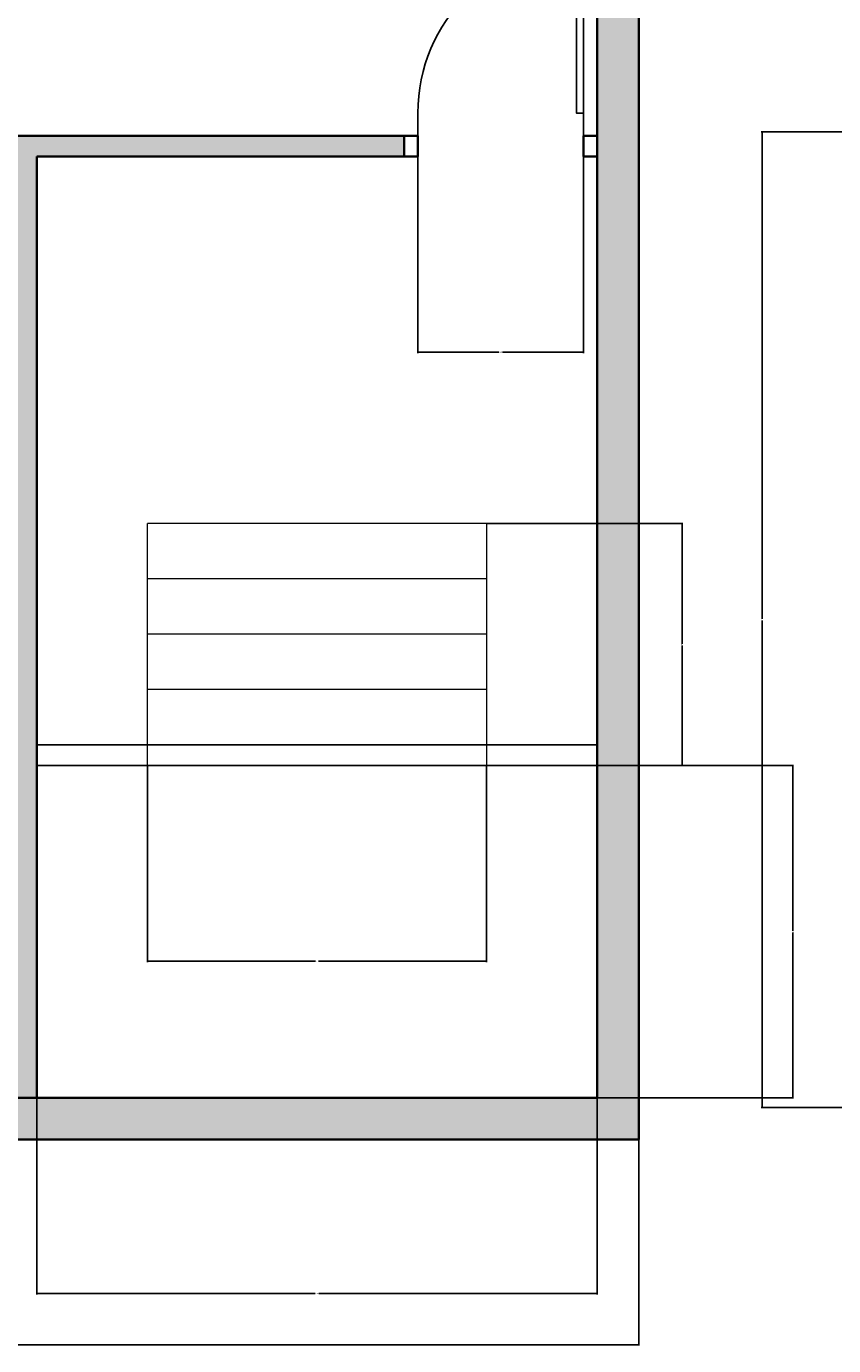
# Model space of a CAD drawing. Units: inches. Extents: x 1563 to 2428, y 777 to 1464.
# Tile 2 of 11: x 1832 to 2007, y 777 to 1063. Entities that reach past the tile are written whole.
import ezdxf

# ---------------------------------------------------------------- set-up
doc = ezdxf.new("R2010")
doc.units = ezdxf.units.IN
for name, color, linetype, lineweight in [('A-ANNO-DIMS', 2, 'Continuous', 18), ('A-DOOR', 4, 'Continuous', 25), ('A-FLOR-EDGE', 7, 'Continuous', 25), ('A-FLOR-STRS', 7, 'Continuous', 18), ('A-WALL', 7, 'Continuous', 35), ('A-WALL-PATT', 8, 'Continuous', 13)]:
    doc.layers.add(name, color=color, linetype=linetype, lineweight=lineweight)
doc.styles.get("Standard").update_dxf_attribs({"font": 'arial.ttf'})
doc.dimstyles.get("Standard").update_dxf_attribs({"dimtxt": 0.18, "dimasz": 0.18, "dimexe": 0.18, "dimexo": 0.0625, "dimgap": 0.09, "dimtad": 0, "dimtih": 1, "dimtoh": 1, "dimdec": 4, "dimzin": 0, "dimdsep": 46, "dimtxsty": 'Standard', "dimcen": 0.09, "dimadec": 0, "dimazin": 0, "dimtfac": 1, "dimtdec": 4, "dimtofl": 0, "dimtmove": 0, "dimatfit": 3, "dimfxl": 1, "dimtolj": 1, "dimtzin": 0, "dimarcsym": 0})

# ---------------------------------------------------------------- blocks, each defined once
blk = doc.blocks.new('*U3')
for p, q in [((0, 0), (0, -6)), ((-40, 0), (-40, -6))]:
    blk.add_line(p, q)
blk.add_lwpolyline([(0, 0), (0, 40), (-1.75, 40), (-1.75, 0)], close=True)
blk.add_arc((0, 0), 40, 90, 180)
blk = doc.blocks.new('*D48')
at = {"layer": 'A-ANNO-DIMS', "color": 0, "lineweight": -2, "transparency": 16777216}
for p, q in [((1605.11, 821.37), (1605.11, 776.74)), ((1965.11, 821.37), (1965.11, 776.74)), ((1605.29, 776.92), (1784.82, 776.92)), ((1964.93, 776.92), (1785.39, 776.92))]:
    blk.add_line(p, q, dxfattribs=at)
at = {"layer": 'A-ANNO-DIMS', "color": 0, "transparency": 16777216}
for points in [[(1605.29, 776.95), (1605.29, 776.89), (1605.11, 776.92)], [(1964.93, 776.95), (1964.93, 776.89), (1965.11, 776.92)]]:
    blk.add_solid(points, dxfattribs=at)
at = {"layer": 'Defpoints', "color": 0, "transparency": 16777216}
for p in [(1605.11, 821.43), (1965.11, 821.43), (1965.11, 776.92)]:
    blk.add_point(p, dxfattribs=at)
at = {"layer": 'A-ANNO-DIMS', "color": 0, "transparency": 16777216, "insert": (1785.11, 776.92), "char_height": 0.18, "attachment_point": 5}
blk.add_mtext('\\A1;360', dxfattribs=at)
blk = doc.blocks.new('*D61')
at = {"layer": 'A-ANNO-DIMS', "color": 0, "lineweight": -2, "transparency": 16777216}
for p, q in [((1834.61, 830.37), (1834.61, 787.85)), ((1956.11, 830.37), (1956.11, 787.85)), ((1834.79, 788.03), (1894.97, 788.03)), ((1955.93, 788.03), (1895.74, 788.03))]:
    blk.add_line(p, q, dxfattribs=at)
at = {"layer": 'A-ANNO-DIMS', "color": 0, "transparency": 16777216}
for points in [[(1834.79, 788.06), (1834.79, 788), (1834.61, 788.03)], [(1955.93, 788.06), (1955.93, 788), (1956.11, 788.03)]]:
    blk.add_solid(points, dxfattribs=at)
at = {"layer": 'Defpoints', "color": 0, "transparency": 16777216}
for p in [(1834.61, 830.43), (1956.11, 830.43), (1834.61, 788.03)]:
    blk.add_point(p, dxfattribs=at)
at = {"layer": 'A-ANNO-DIMS', "color": 0, "transparency": 16777216, "insert": (1895.36, 788.03), "char_height": 0.18, "attachment_point": 5}
blk.add_mtext('\\A1;121.5', dxfattribs=at)
blk = doc.blocks.new('*D62')
at = {"layer": 'A-ANNO-DIMS', "color": 0, "lineweight": -2, "transparency": 16777216}
for p, q in [((1956.17, 902.43), (1998.69, 902.43)), ((1998.51, 902.25), (1998.51, 866.61)), ((1998.51, 830.61), (1998.51, 866.25)), ((1956.17, 830.43), (1998.69, 830.43))]:
    blk.add_line(p, q, dxfattribs=at)
at = {"layer": 'A-ANNO-DIMS', "color": 0, "transparency": 16777216}
for points in [[(1998.48, 902.25), (1998.54, 902.25), (1998.51, 902.43)], [(1998.48, 830.61), (1998.54, 830.61), (1998.51, 830.43)]]:
    blk.add_solid(points, dxfattribs=at)
at = {"layer": 'Defpoints', "color": 0, "transparency": 16777216}
for p in [(1956.11, 902.43), (1956.11, 830.43), (1998.51, 830.43)]:
    blk.add_point(p, dxfattribs=at)
at = {"layer": 'A-ANNO-DIMS', "color": 0, "transparency": 16777216, "insert": (1998.51, 866.43), "char_height": 0.18, "attachment_point": 5}
blk.add_mtext('\\A1;72', dxfattribs=at)
blk = doc.blocks.new('*D63')
at = {"layer": 'A-ANNO-DIMS', "color": 0, "lineweight": -2, "transparency": 16777216}
for p, q in [((1917.22, 1034.37), (1917.22, 991.85)), ((1953.11, 1034.37), (1953.11, 991.85)), ((1917.4, 992.03), (1934.77, 992.03)), ((1952.93, 992.03), (1935.56, 992.03))]:
    blk.add_line(p, q, dxfattribs=at)
at = {"layer": 'A-ANNO-DIMS', "color": 0, "transparency": 16777216}
for points in [[(1917.4, 992.06), (1917.4, 992), (1917.22, 992.03)], [(1952.93, 992.06), (1952.93, 992), (1953.11, 992.03)]]:
    blk.add_solid(points, dxfattribs=at)
at = {"layer": 'Defpoints', "color": 0, "transparency": 16777216}
for p in [(1917.22, 1034.43), (1953.11, 1034.43), (1917.22, 992.03)]:
    blk.add_point(p, dxfattribs=at)
at = {"layer": 'A-ANNO-DIMS', "color": 0, "transparency": 16777216, "insert": (1935.16, 992.03), "char_height": 0.18, "attachment_point": 5}
blk.add_mtext('\\A1;35.88', dxfattribs=at)
blk = doc.blocks.new('*D69')
at = {"layer": 'A-ANNO-DIMS', "color": 0, "lineweight": -2, "transparency": 16777216}
for p, q in [((1858.61, 902.37), (1858.61, 859.85)), ((1932.11, 902.37), (1932.11, 859.85)), ((1858.79, 860.03), (1895.03, 860.03)), ((1931.93, 860.03), (1895.68, 860.03))]:
    blk.add_line(p, q, dxfattribs=at)
at = {"layer": 'A-ANNO-DIMS', "color": 0, "transparency": 16777216}
for points in [[(1858.79, 860.06), (1858.79, 860), (1858.61, 860.03)], [(1931.93, 860.06), (1931.93, 860), (1932.11, 860.03)]]:
    blk.add_solid(points, dxfattribs=at)
at = {"layer": 'Defpoints', "color": 0, "transparency": 16777216}
for p in [(1858.61, 902.43), (1932.11, 902.43), (1858.61, 860.03)]:
    blk.add_point(p, dxfattribs=at)
at = {"layer": 'A-ANNO-DIMS', "color": 0, "transparency": 16777216, "insert": (1895.36, 860.03), "char_height": 0.18, "attachment_point": 5}
blk.add_mtext('\\A1;73.5', dxfattribs=at)
blk = doc.blocks.new('*D70')
at = {"layer": 'A-ANNO-DIMS', "color": 0, "lineweight": -2, "transparency": 16777216}
for p, q in [((1932.17, 954.93), (1974.69, 954.93)), ((1974.51, 954.75), (1974.51, 928.86)), ((1974.51, 902.61), (1974.51, 928.5)), ((1932.17, 902.43), (1974.69, 902.43))]:
    blk.add_line(p, q, dxfattribs=at)
at = {"layer": 'A-ANNO-DIMS', "color": 0, "transparency": 16777216}
for points in [[(1974.48, 954.75), (1974.54, 954.75), (1974.51, 954.93)], [(1974.48, 902.61), (1974.54, 902.61), (1974.51, 902.43)]]:
    blk.add_solid(points, dxfattribs=at)
at = {"layer": 'Defpoints', "color": 0, "transparency": 16777216}
for p in [(1932.11, 954.93), (1932.11, 902.43), (1974.51, 902.43)]:
    blk.add_point(p, dxfattribs=at)
at = {"layer": 'A-ANNO-DIMS', "color": 0, "transparency": 16777216, "insert": (1974.51, 928.68), "char_height": 0.18, "attachment_point": 5}
blk.add_mtext('\\A1;52.5', dxfattribs=at)
blk = doc.blocks.new('*D78')
at = {"layer": 'A-ANNO-DIMS', "color": 0, "lineweight": -2, "transparency": 16777216}
for p, q in [((2034.21, 1039.82), (1991.69, 1039.82)), ((1991.87, 1039.64), (1991.87, 934.26)), ((1991.87, 828.5), (1991.87, 933.89)), ((2034.21, 828.32), (1991.69, 828.32))]:
    blk.add_line(p, q, dxfattribs=at)
at = {"layer": 'A-ANNO-DIMS', "color": 0, "transparency": 16777216}
for points in [[(1991.84, 1039.64), (1991.9, 1039.64), (1991.87, 1039.82)], [(1991.84, 828.5), (1991.9, 828.5), (1991.87, 828.32)]]:
    blk.add_solid(points, dxfattribs=at)
at = {"layer": 'Defpoints', "color": 0, "transparency": 16777216}
for p in [(1991.87, 1039.82), (2034.27, 1039.82), (2034.27, 828.32)]:
    blk.add_point(p, dxfattribs=at)
at = {"layer": 'A-ANNO-DIMS', "color": 0, "transparency": 16777216, "insert": (1991.87, 934.07), "char_height": 0.18, "attachment_point": 5}
blk.add_mtext('\\A1;211.5', dxfattribs=at)

msp = doc.modelspace()

# ---------------------------------------------------------------- hatches: boundary and pattern name
at = {"layer": 'A-WALL-PATT'}
h = msp.add_hatch(color=256, dxfattribs=at)
h.dxf.hatch_style = 1
h.paths.add_polyline_path([(1965.105, 1421.428), (1605.105, 1421.428), (1605.105, 821.428), (1965.105, 821.428)])
h.paths.add_polyline_path([(1614.105, 1199.428), (1704.105, 1199.428), (1738.605, 1199.428), (1738.605, 1251.928), (1734.105, 1251.928), (1734.105, 1203.928), (1704.105, 1203.928), (1614.105, 1203.928), (1614.105, 1335.928), (1665.105, 1335.928), (1665.105, 1340.428), (1614.105, 1340.428), (1614.105, 1412.428), (1704.105, 1412.428), (1704.105, 1340.428), (1701.105, 1340.428), (1701.105, 1335.928), (1704.105, 1335.928), (1768.605, 1335.928), (1768.605, 1340.428), (1708.605, 1340.428), (1708.605, 1412.428), (1807.605, 1412.428), (1807.605, 1340.428), (1804.605, 1340.428), (1804.605, 1335.928), (1807.605, 1335.928), (1807.605, 1275.928), (1815.105, 1275.928), (1815.105, 1280.428), (1812.105, 1280.428), (1812.105, 1412.428), (1956.105, 1412.428), (1956.105, 1280.428), (1854.105, 1280.428), (1854.105, 1275.928), (1956.105, 1275.928), (1956.105, 830.428), (1614.105, 830.428)], flags=16)
h.paths.add_polyline_path([(1917.224, 1038.928), (1917.224, 1043.846, -0.4014527), (1951.591, 1079.751), (1951.591, 1079.786), (1953.163, 1079.786), (1953.163, 1043.846), (1953.163, 1038.455), (1953.105, 1034.428), (1953.105, 1038.928), (1953.163, 1043.846), (1951.591, 1043.846), (1951.591, 1079.751, 0.4014527), (1917.224, 1043.846), (1917.224, 1038.455), (1917.224, 1034.428), (1834.605, 1034.428), (1834.605, 906.928), (1858.605, 906.928), (1858.605, 954.928), (1932.105, 954.928), (1932.105, 902.428), (1834.605, 902.428), (1834.605, 1034.428), (1914.224, 1034.428), (1914.224, 1038.928)], flags=0)
edge = h.paths.add_edge_path(flags=0)
edge.add_ellipse((1674.345, 1004.483), major_axis=(1.48, 0), ratio=0.8423039, start_angle=90, end_angle=180, ccw=False)
edge.add_line((1674.345, 1005.73), (1674.921, 1005.73))
edge.add_ellipse((2202.617, 985.642), major_axis=(528.234, 0), ratio=0.8423039, start_angle=176.34957, end_angle=177.82005, ccw=False)
edge.add_ellipse((1739.278, 760.804), major_axis=(-313.308, 0), ratio=0.8423039, start_angle=-77.87403, end_angle=-76.21947, ccw=False)
edge.add_ellipse((1739.278, 767.659), major_axis=(305.303, 0), ratio=0.8423039, start_angle=100.20954, end_angle=102.44463, ccw=False)
edge.add_ellipse((1659.357, 1231.328), major_axis=(250.96, 0), ratio=0.8423039, start_angle=-80.74343, end_angle=-77.44507)
edge.add_line((1705.625, 1023.567), (1711.685, 1026.918))
edge.add_ellipse((1711.754, 1026.21), major_axis=(0.74, 0), ratio=0.8423039, start_angle=52.06687, end_angle=90, ccw=False)
edge.add_line((1712.16, 1026.731), (1717.882, 1023.567))
edge.add_ellipse((1764.151, 1231.328), major_axis=(250.96, 0), ratio=0.8423039, start_angle=257.44507, end_angle=260.74343)
edge.add_ellipse((1684.229, 767.659), major_axis=(305.303, 0), ratio=0.8423039, start_angle=77.55537, end_angle=79.79046, ccw=False)
edge.add_ellipse((1684.229, 760.804), major_axis=(-313.308, 0), ratio=0.8423039, start_angle=256.21947, end_angle=257.87403, ccw=False)
edge.add_ellipse((1220.891, 985.642), major_axis=(-528.234, 0), ratio=0.8423039, start_angle=182.17995, end_angle=183.65043, ccw=False)
edge.add_line((1748.586, 1005.73), (1749.162, 1005.73))
edge.add_ellipse((1749.162, 1004.483), major_axis=(-1.48, 0), ratio=0.8423039, start_angle=180, end_angle=270, ccw=False)
edge.add_line((1750.642, 1004.483), (1750.642, 980.28))
edge.add_ellipse((1749.162, 980.28), major_axis=(1.48, 0), ratio=0.8423039, start_angle=270, end_angle=360, ccw=False)
edge.add_ellipse((-8843.864, 962.352), major_axis=(10593.026, 0), ratio=0.84230387, start_angle=-0.3241203, end_angle=0.0902291, ccw=False)
edge.add_ellipse((-8843.864, 962.352), major_axis=(10593.026, 0), ratio=0.84230387, start_angle=-0.3838668, end_angle=-0.3241203, ccw=False)
edge.add_ellipse((1749.162, 890.136), major_axis=(1.48, 0), ratio=0.8423039, start_angle=0, end_angle=90, ccw=False)
edge.add_line((1750.642, 890.136), (1750.642, 865.933))
edge.add_ellipse((1749.162, 865.933), major_axis=(1.48, 0), ratio=0.8423039, start_angle=270, end_angle=360, ccw=False)
edge.add_line((1749.162, 864.686), (1748.528, 864.686))
edge.add_ellipse((-8843.864, 962.352), major_axis=(10593.026, 0), ratio=0.84230387, start_angle=-0.6186432, end_angle=-0.5282715, ccw=False)
edge.add_ellipse((1747.592, 846.206), major_axis=(-2.22, 0), ratio=0.8423039, start_angle=179.37176, end_angle=248.46476, ccw=False)
edge.add_ellipse((-8844.604, 962.352), major_axis=(-10595.313, 0), ratio=0.842303864, start_angle=179.3534459, end_angle=179.3717628, ccw=False)
edge.add_ellipse((1744.512, 842.854), major_axis=(-5.246, 0), ratio=0.8423039, start_angle=90, end_angle=179.35345, ccw=False)
edge.add_line((1744.512, 838.435), (1678.995, 838.435))
edge.add_ellipse((1678.995, 842.854), major_axis=(5.246, 0), ratio=0.8423039, start_angle=180.64655, end_angle=270, ccw=False)
edge.add_ellipse((12268.111, 962.352), major_axis=(-10595.313, 0), ratio=0.84230387, start_angle=0.6282372, end_angle=0.6465541, ccw=False)
edge.add_ellipse((1675.916, 846.206), major_axis=(-2.22, 0), ratio=0.8423039, start_angle=-68.46476, end_angle=0.62824, ccw=False)
edge.add_ellipse((12267.371, 962.352), major_axis=(-10593.026, 0), ratio=0.84230387, start_angle=0.5282715, end_angle=0.6465541, ccw=False)
edge.add_line((1674.98, 864.686), (1674.345, 864.686))
edge.add_ellipse((1674.345, 865.933), major_axis=(-1.48, 0), ratio=0.8423039, start_angle=0, end_angle=90, ccw=False)
edge.add_line((1672.865, 865.933), (1672.865, 890.136))
edge.add_ellipse((1674.345, 890.136), major_axis=(1.48, 0), ratio=0.8423039, start_angle=90, end_angle=180, ccw=False)
edge.add_ellipse((12267.371, 962.352), major_axis=(-10593.026, 0), ratio=0.84230387, start_angle=0.3241203, end_angle=0.3838668, ccw=False)
edge.add_ellipse((12267.371, 962.352), major_axis=(-10593.026, 0), ratio=0.84230387, start_angle=-0.0902291, end_angle=0.3241203, ccw=False)
edge.add_ellipse((1674.345, 980.28), major_axis=(-1.48, 0), ratio=0.8423039, start_angle=0, end_angle=90, ccw=False)
edge.add_line((1672.865, 980.28), (1672.865, 1004.483))
h.paths.add_polyline_path([(1622.542, 1135.584), (1648.534, 1136.233), (1648.683, 1130.234), (1647.126, 1130.196), (1648.323, 1082.21), (1649.88, 1082.249), (1650.03, 1076.251), (1624.038, 1075.603, -0.266667)], flags=0)
edge = h.paths.add_edge_path(flags=0)
edge.add_line((1694.584, 990.705), (1700.334, 994.711))
edge.add_line((1700.334, 994.711), (1702.248, 994.711))
edge.add_line((1702.248, 994.711), (1702.248, 997.061))
edge.add_ellipse((1758.417, 997.061), major_axis=(56.169, 0), ratio=0.8423039, start_angle=150.56143, end_angle=180, ccw=False)
edge.add_ellipse((1665.091, 997.061), major_axis=(-56.169, 0), ratio=0.8423039, start_angle=180, end_angle=209.43857, ccw=False)
edge.add_line((1721.26, 997.061), (1721.26, 994.711))
edge.add_line((1721.26, 994.711), (1723.174, 994.711))
edge.add_line((1723.174, 994.711), (1728.923, 990.705))
edge.add_line((1728.923, 990.705), (1728.923, 975.895))
edge.add_ellipse((1725.091, 976.043), major_axis=(0.357, 6.34), ratio=0.6038336, start_angle=106.34259, end_angle=270.99799, ccw=False)
edge.add_line((1721.26, 975.15), (1721.26, 997.061))
edge.add_ellipse((1665.091, 997.061), major_axis=(-56.169, 0), ratio=0.8423039, start_angle=180, end_angle=209.43857)
edge.add_ellipse((1758.417, 997.061), major_axis=(56.169, 0), ratio=0.8423039, start_angle=150.56143, end_angle=180)
edge.add_line((1702.248, 997.061), (1702.248, 975.15))
edge.add_ellipse((1698.416, 976.043), major_axis=(-0.357, 6.34), ratio=0.6038336, start_angle=89.00201, end_angle=253.65741, ccw=False)
edge.add_line((1694.584, 975.895), (1694.584, 990.705))
edge = h.paths.add_edge_path(flags=0)
edge.add_line((1675.832, 952.075), (1679.883, 938.848))
edge.add_ellipse((5378.107, 931.045), major_axis=(-3698.236, 0), ratio=0.84230387, start_angle=-0.120897, end_angle=0.364076)
edge.add_line((1679.976, 907.545), (1676.149, 892.52))
edge.add_ellipse((12267.371, 962.352), major_axis=(10591.546, 0), ratio=0.84230387, start_angle=180.3241656, end_angle=180.3777642, ccw=False)
edge.add_ellipse((12267.371, 962.352), major_axis=(10591.546, 0), ratio=0.84230387, start_angle=180.0555943, end_angle=180.3241656, ccw=False)
edge = h.paths.add_edge_path(flags=0)
edge.add_ellipse((1706.366, 891.542), major_axis=(81.773, 0), ratio=0.8423039, start_angle=94.27742, end_angle=111.83495, ccw=False)
edge.add_line((1701.225, 960.283), (1722.283, 960.283))
edge.add_ellipse((1717.141, 891.542), major_axis=(-81.773, 0), ratio=0.8423039, start_angle=248.16505, end_angle=265.72258, ccw=False)
edge.add_line((1743.29, 956.803), (1741.105, 940.427))
edge.add_ellipse((1714.553, 877.238), major_axis=(79.58, 0), ratio=0.8423039, start_angle=67.20809, end_angle=85.12993)
edge.add_line((1720.25, 944.097), (1703.258, 944.097))
edge.add_ellipse((1708.954, 877.238), major_axis=(79.58, 0), ratio=0.8423039, start_angle=94.87007, end_angle=112.79191)
edge.add_line((1682.403, 940.427), (1680.218, 956.803))
h.paths.add_polyline_path([(1664.992, 1093.991), (1664.992, 1123.991), (1724.992, 1123.991), (1724.992, 1093.991)], flags=0)
h.paths.add_polyline_path([(1716.588, 1099.729), (1715.404, 1099.805), (1715.021, 1099.823), (1716.177, 1099.758)], flags=0)
h.paths.add_polyline_path([(1711.325, 1103.757), (1712.167, 1103.706), (1713.009, 1103.642), (1713.84, 1103.566), (1715.041, 1103.439), (1716.532, 1103.244), (1717.793, 1103.048), (1718.876, 1102.854), (1719.676, 1102.699), (1720.157, 1102.605), (1720.632, 1102.513), (1721.109, 1102.424), (1721.595, 1102.339), (1722.088, 1102.264), (1722.585, 1102.205), (1723.082, 1102.17), (1723.575, 1102.164), (1724.321, 1102.211), (1724.533, 1102.268), (1723.842, 1102.16), (1722.864, 1102.172), (1721.894, 1102.287), (1720.935, 1102.454), (1720.157, 1102.605), (1719.676, 1102.699), (1719.18, 1102.795), (1718.66, 1102.892), (1718.109, 1102.991), (1717.517, 1103.091), (1716.876, 1103.191), (1716.179, 1103.29), (1715.435, 1103.387), (1714.652, 1103.48), (1713.84, 1103.566), (1713.009, 1103.642), (1712.167, 1103.706), (1711.325, 1103.757), (1710.492, 1103.791), (1709.676, 1103.806), (1708.873, 1103.805), (1707.707, 1103.78), (1707.292, 1103.757), (1708.499, 1103.805), (1710.086, 1103.807)], flags=0)
h.paths.add_polyline_path([(1713.959, 1106.591), (1714.651, 1106.624), (1715.279, 1106.674), (1715.852, 1106.736), (1716.373, 1106.807), (1716.851, 1106.885), (1717.289, 1106.966), (1717.696, 1107.046), (1718.341, 1107.178), (1719.173, 1107.331), (1720.169, 1107.421), (1721.131, 1107.383), (1722.032, 1107.286), (1722.934, 1107.152), (1723.887, 1106.983), (1724.746, 1106.795), (1724.72, 1106.798), (1724.663, 1106.807), (1724.241, 1106.906), (1724.159, 1106.924), (1723.885, 1106.979), (1723.546, 1107.044), (1723.157, 1107.113), (1722.732, 1107.182), (1722.284, 1107.249), (1721.827, 1107.308), (1721.375, 1107.357), (1720.942, 1107.391), (1720.539, 1107.406), (1720.162, 1107.405), (1719.804, 1107.388), (1719.459, 1107.357), (1719.12, 1107.314), (1718.781, 1107.259), (1718.435, 1107.195), (1718.076, 1107.124), (1717.402, 1106.986), (1716.59, 1106.837), (1715.56, 1106.696), (1714.317, 1106.598)], flags=0)
h.paths.add_polyline_path([(1708.692, 1110.124), (1709.455, 1110.13), (1710.147, 1110.149), (1710.772, 1110.18), (1711.334, 1110.224), (1711.836, 1110.28), (1712.283, 1110.349), (1712.678, 1110.43), (1713.026, 1110.524), (1713.33, 1110.63), (1713.596, 1110.746), (1713.832, 1110.87), (1714.042, 1110.999), (1714.234, 1111.131), (1714.413, 1111.264), (1714.586, 1111.396), (1715.065, 1111.75), (1715.879, 1112.11), (1716.842, 1112.224), (1717.903, 1112.165), (1719.048, 1111.965), (1719.867, 1111.736), (1720.686, 1111.487), (1721.596, 1111.22), (1721.917, 1111.136), (1721.028, 1111.383), (1720.222, 1111.628), (1719.815, 1111.75), (1719.434, 1111.857), (1719.054, 1111.951), (1718.672, 1112.031), (1718.292, 1112.097), (1717.918, 1112.149), (1717.554, 1112.185), (1717.204, 1112.204), (1716.871, 1112.206), (1716.559, 1112.191), (1716.271, 1112.156), (1716.006, 1112.105), (1715.761, 1112.038), (1715.534, 1111.957), (1715.323, 1111.864), (1715.125, 1111.759), (1714.937, 1111.645), (1714.759, 1111.524), (1714.586, 1111.396), (1714.413, 1111.264), (1714.003, 1110.96), (1713.331, 1110.606), (1712.501, 1110.382), (1711.61, 1110.245), (1710.489, 1110.158), (1709.111, 1110.121)], flags=0)
h.paths.add_polyline_path([(1707.127, 1113.075), (1707.639, 1113.025), (1708.092, 1112.991), (1708.49, 1112.975), (1708.836, 1112.977), (1709.135, 1112.996), (1709.392, 1113.032), (1709.612, 1113.084), (1709.798, 1113.15), (1709.957, 1113.23), (1710.092, 1113.324), (1710.208, 1113.431), (1710.304, 1113.554), (1710.379, 1113.698), (1710.434, 1113.866), (1710.467, 1114.062), (1710.477, 1114.289), (1710.463, 1114.553), (1710.426, 1114.857), (1710.364, 1115.202), (1710.282, 1115.58), (1710.184, 1115.98), (1710.076, 1116.391), (1709.961, 1116.801), (1709.844, 1117.201), (1709.731, 1117.579), (1709.626, 1117.924), (1709.532, 1118.228), (1709.454, 1118.493), (1709.392, 1118.723), (1709.351, 1118.924), (1709.293, 1119.435), (1709.831, 1119.942), (1710.705, 1120.121), (1711.507, 1119.898), (1712.224, 1119.567), (1713.189, 1119.016), (1713.529, 1118.804), (1712.958, 1119.148), (1712.468, 1119.428), (1712.046, 1119.649), (1711.683, 1119.817), (1711.366, 1119.937), (1711.084, 1120.016), (1710.826, 1120.057), (1710.582, 1120.067), (1710.354, 1120.049), (1710.142, 1120.006), (1709.951, 1119.941), (1709.781, 1119.857), (1709.635, 1119.757), (1709.516, 1119.645), (1709.426, 1119.524), (1709.366, 1119.395), (1709.335, 1119.255), (1709.331, 1119.1), (1709.351, 1118.924), (1709.392, 1118.723), (1709.454, 1118.493), (1709.52, 1118.268), (1709.799, 1117.356), (1710.028, 1116.57), (1710.245, 1115.749), (1710.45, 1114.804), (1710.477, 1114.289), (1710.448, 1113.654), (1709.908, 1113.153), (1709.165, 1112.979), (1708.318, 1112.974), (1707.448, 1113.039)], flags=0)
h.paths.add_polyline_path([(1700.892, 1119.857), (1701.604, 1119.819), (1702.196, 1119.805), (1702.683, 1119.813), (1703.076, 1119.841), (1703.387, 1119.887), (1703.63, 1119.951), (1703.816, 1120.03), (1703.959, 1120.124), (1704.069, 1120.23), (1704.15, 1120.346), (1704.204, 1120.47), (1704.234, 1120.599), (1704.242, 1120.731), (1704.231, 1120.864), (1704.202, 1120.996), (1704.159, 1121.124), (1704.103, 1121.246), (1704.039, 1121.362), (1703.97, 1121.474), (1703.901, 1121.582), (1703.834, 1121.687), (1703.775, 1121.79), (1703.564, 1122.226), (1704.048, 1122.698), (1704.756, 1122.769), (1705.49, 1122.723), (1706.24, 1122.641), (1706.547, 1122.601), (1706.092, 1122.657), (1705.695, 1122.701), (1705.348, 1122.732), (1705.049, 1122.751), (1704.792, 1122.757), (1704.573, 1122.751), (1704.386, 1122.732), (1704.227, 1122.701), (1704.092, 1122.657), (1703.977, 1122.601), (1703.88, 1122.534), (1703.802, 1122.458), (1703.742, 1122.374), (1703.702, 1122.284), (1703.68, 1122.188), (1703.677, 1122.09), (1703.692, 1121.991), (1703.726, 1121.89), (1703.769, 1121.802), (1704.039, 1121.362), (1704.301, 1120.887), (1704.133, 1120.165), (1703.43, 1119.866), (1702.481, 1119.798), (1701.306, 1119.827)], flags=0)
edge = h.paths.add_edge_path(flags=0)
edge.add_ellipse((1711.754, 1009.752), major_axis=(-147.018, 0), ratio=0.8423039, start_angle=76.40187, end_angle=103.59813)
edge.add_line((1741.105, 888.411), (1741.105, 869.587))
edge.add_ellipse((1711.754, 990.928), major_axis=(-147.018, 0), ratio=0.8423039, start_angle=76.40187, end_angle=103.59813, ccw=False)
edge.add_line((1682.403, 869.587), (1682.403, 888.411))
edge = h.paths.add_edge_path(flags=0)
edge.add_ellipse((-8843.864, 962.352), major_axis=(-10591.546, 0), ratio=0.84230387, start_angle=179.6758344, end_angle=179.9444057, ccw=False)
edge.add_ellipse((-8843.864, 962.352), major_axis=(-10591.546, 0), ratio=0.84230387, start_angle=179.6222358, end_angle=179.6758344, ccw=False)
edge.add_line((1747.358, 892.52), (1743.531, 907.545))
edge.add_ellipse((-1954.6, 931.045), major_axis=(3698.236, 0), ratio=0.84230387, start_angle=-0.364076, end_angle=0.120897)
edge.add_line((1743.625, 938.848), (1747.676, 952.075))
h.paths.add_polyline_path([(1637.931, 1162.087), (1637.931, 1188.087, -0.1904762), (1721.931, 1188.087), (1721.931, 1162.087), (1715.931, 1162.087), (1715.931, 1163.644), (1643.931, 1163.644), (1643.931, 1162.087)], flags=0)
h.paths.add_polyline_path([(1667.931, 1189.491, -0.0496282), (1691.931, 1189.491), (1691.931, 1182.705), (1667.931, 1182.705)], flags=0)
edge = h.paths.add_edge_path(flags=0)
edge.add_ellipse((1685.362, 859.825), major_axis=(-2.96, 0), ratio=0.8423039, start_angle=-90, end_angle=0, ccw=False)
edge.add_line((1685.362, 862.318), (1738.145, 862.318))
edge.add_ellipse((1738.145, 859.825), major_axis=(2.96, 0), ratio=0.8423039, start_angle=0, end_angle=90, ccw=False)
edge.add_line((1741.105, 859.825), (1741.105, 840.361))
edge.add_line((1741.105, 840.361), (1682.403, 840.361))
edge.add_line((1682.403, 840.361), (1682.403, 859.825))
h.paths.add_polyline_path([(1777.486, 1164.853), (1777.486, 1180.853), (1778.486, 1181.01), (1778.486, 1164.697)], flags=0)
h.paths.add_polyline_path([(1786.986, 1154.853), (1786.986, 1163.369), (1778.986, 1164.619), (1778.986, 1181.088), (1786.986, 1182.338), (1786.986, 1190.853), (1799.502, 1190.853), (1800.752, 1198.853), (1817.221, 1198.853), (1818.471, 1190.853), (1827.502, 1190.853), (1828.752, 1198.853), (1845.221, 1198.853), (1846.471, 1190.853), (1858.986, 1190.853), (1858.986, 1182.338), (1866.986, 1181.088), (1866.986, 1164.619), (1858.986, 1163.369), (1858.986, 1154.853), (1846.471, 1154.853), (1845.221, 1146.853), (1828.752, 1146.853), (1827.502, 1154.853), (1818.471, 1154.853), (1817.221, 1146.853), (1800.752, 1146.853), (1799.502, 1154.853)], flags=0)
h.paths.add_polyline_path([(1800.986, 1145.353), (1800.83, 1146.353), (1817.143, 1146.353), (1816.986, 1145.353)], flags=0)
h.paths.add_polyline_path([(1851.408, 1167.858), (1852.086, 1167.738), (1852.744, 1167.621), (1853.388, 1167.506), (1854.028, 1167.395), (1854.67, 1167.289), (1855.313, 1167.195), (1855.952, 1167.122), (1856.585, 1167.077), (1857.209, 1167.07), (1858.147, 1167.128), (1858.413, 1167.2), (1857.547, 1167.066), (1856.312, 1167.08), (1855.07, 1167.223), (1854.028, 1167.395), (1853.388, 1167.506), (1852.744, 1167.621), (1852.086, 1167.738), (1851.408, 1167.858), (1850.288, 1168.052), (1849.956, 1168.104), (1850.701, 1167.98)], flags=0)
h.paths.add_polyline_path([(1845.435, 1172.646), (1846.222, 1172.707), (1846.941, 1172.785), (1847.601, 1172.874), (1848.21, 1172.971), (1848.777, 1173.072), (1849.311, 1173.173), (1850.14, 1173.331), (1851.063, 1173.483), (1852.014, 1173.591), (1853.012, 1173.633), (1854.075, 1173.594), (1855.251, 1173.473), (1856.4, 1173.306), (1857.391, 1173.132), (1857.945, 1173.02), (1858.196, 1172.965), (1858.595, 1172.871), (1858.575, 1172.874), (1858.49, 1172.894), (1858.371, 1172.924), (1858.196, 1172.965), (1857.945, 1173.02), (1857.602, 1173.089), (1857.177, 1173.17), (1856.687, 1173.256), (1856.148, 1173.343), (1855.575, 1173.426), (1854.986, 1173.5), (1854.395, 1173.561), (1853.82, 1173.603), (1853.272, 1173.623), (1852.749, 1173.622), (1852.247, 1173.6), (1851.757, 1173.562), (1851.276, 1173.507), (1850.796, 1173.439), (1850.313, 1173.359), (1849.82, 1173.27), (1849.311, 1173.173), (1848.421, 1173.005), (1847.25, 1172.818), (1845.826, 1172.665)], flags=0)
h.paths.add_polyline_path([(1840.587, 1177.09), (1841.289, 1177.145), (1841.916, 1177.215), (1842.475, 1177.301), (1842.969, 1177.403), (1843.403, 1177.52), (1843.783, 1177.652), (1844.117, 1177.797), (1844.411, 1177.952), (1844.674, 1178.114), (1844.914, 1178.279), (1845.138, 1178.446), (1845.644, 1178.831), (1846.285, 1179.221), (1847.125, 1179.521), (1847.998, 1179.624), (1848.834, 1179.619), (1849.768, 1179.529), (1850.775, 1179.363), (1851.78, 1179.14), (1852.111, 1179.053), (1851.57, 1179.187), (1851.043, 1179.304), (1850.527, 1179.404), (1850.024, 1179.487), (1849.539, 1179.551), (1849.072, 1179.596), (1848.628, 1179.62), (1848.21, 1179.623), (1847.82, 1179.603), (1847.46, 1179.561), (1847.128, 1179.497), (1846.822, 1179.413), (1846.539, 1179.312), (1846.274, 1179.195), (1846.027, 1179.064), (1845.793, 1178.922), (1845.57, 1178.77), (1845.354, 1178.61), (1844.817, 1178.201), (1844.106, 1177.764), (1843.208, 1177.452), (1842.225, 1177.25), (1840.973, 1177.11)], flags=0)
h.paths.add_polyline_path([(1836.67, 1180.646), (1837.236, 1180.603), (1837.734, 1180.584), (1838.166, 1180.586), (1838.54, 1180.611), (1838.861, 1180.655), (1839.136, 1180.72), (1839.369, 1180.803), (1839.568, 1180.903), (1839.736, 1181.02), (1839.881, 1181.152), (1840.001, 1181.299), (1840.095, 1181.456), (1840.164, 1181.624), (1840.204, 1181.8), (1840.217, 1181.981), (1840.2, 1182.166), (1840.153, 1182.353), (1840.076, 1182.541), (1839.973, 1182.728), (1839.851, 1182.916), (1839.716, 1183.103), (1839.572, 1183.291), (1839.427, 1183.478), (1839.033, 1184), (1838.862, 1184.411), (1838.695, 1184.99), (1839.2, 1185.669), (1840.06, 1185.961), (1840.793, 1185.931), (1841.454, 1185.77), (1842.179, 1185.536), (1842.706, 1185.363), (1843.713, 1185.044), (1844.033, 1184.956), (1843.102, 1185.234), (1842.179, 1185.536), (1841.725, 1185.682), (1841.328, 1185.801), (1840.976, 1185.886), (1840.653, 1185.937), (1840.349, 1185.949), (1840.063, 1185.926), (1839.799, 1185.872), (1839.559, 1185.791), (1839.347, 1185.686), (1839.165, 1185.562), (1839.016, 1185.422), (1838.903, 1185.27), (1838.828, 1185.11), (1838.79, 1184.943), (1838.784, 1184.77), (1838.809, 1184.593), (1838.862, 1184.411), (1838.938, 1184.227), (1839.036, 1184.041), (1839.153, 1183.853), (1839.285, 1183.666), (1839.427, 1183.478), (1839.572, 1183.291), (1839.716, 1183.103), (1839.851, 1182.916), (1840.178, 1182.415), (1840.251, 1181.604), (1839.686, 1180.915), (1838.893, 1180.633), (1837.976, 1180.574), (1837.01, 1180.612)], flags=0)
h.paths.add_polyline_path([(1829.867, 1185.622), (1830.475, 1185.631), (1830.966, 1185.666), (1831.355, 1185.724), (1831.658, 1185.804), (1831.891, 1185.903), (1832.07, 1186.02), (1832.207, 1186.152), (1832.308, 1186.297), (1832.376, 1186.452), (1832.414, 1186.614), (1832.424, 1186.779), (1832.41, 1186.946), (1832.374, 1187.11), (1832.32, 1187.27), (1832.25, 1187.422), (1832.17, 1187.568), (1832.084, 1187.708), (1831.997, 1187.843), (1831.914, 1187.974), (1831.839, 1188.102), (1831.614, 1188.57), (1832.036, 1189.169), (1832.801, 1189.319), (1833.589, 1189.3), (1834.44, 1189.223), (1834.736, 1189.187), (1834.239, 1189.241), (1833.807, 1189.28), (1833.433, 1189.304), (1833.111, 1189.312), (1832.837, 1189.304), (1832.604, 1189.28), (1832.405, 1189.241), (1832.236, 1189.187), (1832.092, 1189.117), (1831.971, 1189.033), (1831.873, 1188.938), (1831.799, 1188.832), (1831.748, 1188.719), (1831.721, 1188.601), (1831.717, 1188.478), (1831.736, 1188.353), (1831.779, 1188.228), (1831.839, 1188.102), (1831.914, 1187.974), (1831.997, 1187.843), (1832.084, 1187.708), (1832.387, 1187.216), (1832.456, 1186.393), (1831.916, 1185.871), (1831.195, 1185.682), (1830.221, 1185.613)], flags=0)
h.paths.add_polyline_path([(1828.986, 1145.353), (1828.83, 1146.353), (1845.143, 1146.353), (1844.986, 1145.353)], flags=0)
h.paths.add_polyline_path([(1800.986, 1200.353), (1816.986, 1200.353), (1817.143, 1199.353), (1800.83, 1199.353)], flags=0)
h.paths.add_polyline_path([(1828.986, 1200.353), (1844.986, 1200.353), (1845.143, 1199.353), (1828.83, 1199.353)], flags=0)
h.paths.add_polyline_path([(1867.486, 1181.01), (1868.486, 1180.853), (1868.486, 1164.853), (1867.486, 1164.697)], flags=0)
h.paths.add_polyline_path([(1901.055, 1112.089), (1901.055, 1241.889), (1954.299, 1241.889), (1954.299, 1112.089)], flags=0)
h.paths.add_polyline_path([(1908.544, 1229.408), (1931.009, 1229.408), (1937.23, 1216.927), (1931.009, 1216.927), (1931.009, 1129.562), (1908.544, 1129.562)], flags=0)
h.paths.add_polyline_path([(1699.472, 1381.538), (1701.045, 1381.538), (1701.045, 1345.599), (1699.472, 1345.599)], flags=0)
h.paths.add_polyline_path([(1851.045, 1285.819), (1851.045, 1280.428), (1851.105, 1275.928), (1851.105, 1280.428)], flags=0)
h.paths.add_polyline_path([(1815.105, 1285.819), (1815.105, 1321.758), (1816.678, 1321.758), (1816.678, 1285.819)], flags=0)
h.paths.add_polyline_path([(1745.154, 1343.707, -0.1044693), (1742.568, 1347.148, -0.1176343), (1741.799, 1350.905, -0.1176343), (1742.808, 1354.603, -0.1044693), (1745.61, 1357.871, -0.0900158), (1749.544, 1359.891, -0.0819199), (1754.355, 1360.526, -0.0819199), (1759.115, 1359.583, -0.0900158), (1762.911, 1357.314, -0.1044693), (1765.497, 1353.872, -0.1176343), (1766.266, 1350.116, -0.1176343), (1765.257, 1346.417, -0.1044693), (1762.455, 1343.149, -0.0900158), (1758.521, 1341.13, -0.0819199), (1753.71, 1340.495, -0.0819199), (1748.95, 1341.438, -0.0900158)], flags=0)
h.paths.add_polyline_path([(1745.961, 1344.152, -0.1046782), (1743.517, 1347.257, -0.1186217), (1742.746, 1350.669, -0.1186217), (1743.612, 1354.059, -0.1046782), (1746.143, 1357.094, -0.0895621), (1749.732, 1359.002, -0.0811847), (1754.161, 1359.662, -0.0811847), (1758.57, 1358.877, -0.0895621), (1762.104, 1356.869, -0.1046782), (1764.548, 1353.764, -0.1186217), (1765.319, 1350.351, -0.1186217), (1764.453, 1346.962, -0.1046782), (1761.922, 1343.927, -0.0895621), (1758.333, 1342.019, -0.0811847), (1753.904, 1341.359, -0.0811847), (1749.495, 1342.143, -0.0895621)], flags=0)
h.paths.add_polyline_path([(1748.738, 1346.3, -0.1046075), (1747.125, 1348.343, -0.1182826), (1746.612, 1350.593, -0.1182826), (1747.176, 1352.832, -0.1046075), (1748.833, 1354.838, -0.089718), (1751.19, 1356.103, -0.0814361), (1754.1, 1356.547, -0.0814361), (1756.999, 1356.038, -0.089718), (1759.327, 1354.72, -0.1046075), (1760.94, 1352.678, -0.1182826), (1761.453, 1350.427, -0.1182826), (1760.889, 1348.189, -0.1046075), (1759.232, 1346.183, -0.089718), (1756.875, 1344.917, -0.0814361), (1753.965, 1344.474, -0.0814361), (1751.066, 1344.982, -0.089718)], flags=0)
h.paths.add_polyline_path([(1802.972, 1381.538), (1804.545, 1381.538), (1804.545, 1345.599), (1802.972, 1345.599)], flags=0)
h.paths.add_polyline_path([(1752.533, 1350.51, -1), (1755.533, 1350.51, -1)], flags=0)
h.paths.add_polyline_path([(1753.033, 1350.51, -1), (1755.033, 1350.51, -1)], flags=0)
h.paths.add_polyline_path([(1869.759, 1336.236), (1869.759, 1396.236), (1949.759, 1396.236), (1949.759, 1336.236)], flags=0)
h.paths.add_polyline_path([(1920.159, 1336.236), (1920.159, 1351.436), (1935.359, 1351.436), (1935.359, 1388.236), (1948.559, 1388.236), (1948.559, 1367.436), (1935.359, 1367.436), (1935.359, 1365.036), (1948.559, 1365.036), (1948.559, 1344.236), (1933.359, 1344.236), (1933.359, 1349.436)], flags=0)
h.paths.add_polyline_path([(1938.156, 1328.719, -1), (1952.156, 1328.719, -1)], flags=0)
h.paths.add_polyline_path([(1942.156, 1328.719), (1945.156, 1331.719), (1948.156, 1328.719), (1945.156, 1325.719)], flags=0)
h.paths.add_polyline_path([(1944.156, 1328.719, -1), (1946.156, 1328.719, -1)], flags=0)
h.paths.add_polyline_path([(1914.224, 1038.928), (1614.105, 1038.928), (1614.105, 1034.428), (1830.105, 1034.428), (1830.105, 830.428), (1834.605, 830.428), (1834.605, 1034.428), (1914.224, 1034.428)], flags=0)
h.paths.add_polyline_path([(1956.105, 902.428), (1834.605, 902.428), (1834.605, 830.428), (1956.105, 830.428)], flags=0)
h = msp.add_hatch(color=256, dxfattribs=at)
h.dxf.hatch_style = 1
h.paths.add_polyline_path([(2385.27, 1419.324), (2025.27, 1419.324), (2025.27, 819.324), (2385.27, 819.324)])
h.paths.add_polyline_path([(2034.27, 1410.324), (2112.27, 1410.324), (2112.27, 1257.324), (2116.77, 1257.324), (2116.77, 1410.324), (2376.27, 1410.324), (2376.27, 1218.324), (2158.77, 1218.324), (2158.77, 1213.824), (2376.27, 1213.824), (2376.27, 1117.824), (2280.27, 1117.824), (2280.27, 1174.824), (2275.77, 1174.824), (2275.77, 1113.324), (2376.27, 1113.324), (2376.27, 828.324), (2214.27, 828.324), (2214.27, 1039.824), (2211.27, 1039.824), (2211.27, 828.324), (2034.27, 828.324), (2034.27, 1039.824), (2172.27, 1039.824), (2172.27, 1044.324), (2034.27, 1044.324), (2034.27, 1136.044, -0.0910221), (2034.27, 1152.131), (2034.27, 1213.824), (2116.77, 1213.824), (2116.77, 1218.324), (2034.27, 1218.324)], flags=16)
h.paths.add_polyline_path([(2106.854, 1222.904), (2106.854, 1221.324), (2070.749, 1221.324), (2070.749, 1222.904)], flags=0)
h.paths.add_polyline_path([(2112.405, 1204.123), (2112.405, 1184.897), (2107.968, 1184.897), (2107.968, 1186.049), (2054.728, 1186.049), (2054.728, 1184.897), (2050.292, 1184.897), (2050.292, 1204.123, -0.1904762)], flags=0)
h.paths.add_polyline_path([(2090.222, 1205.162), (2090.222, 1200.143), (2072.475, 1200.143), (2072.475, 1205.162, -0.0496282)], flags=0)
h.paths.add_polyline_path([(2154.296, 1259.846), (2155.876, 1259.846), (2155.876, 1223.74), (2154.296, 1223.74)], flags=0)
h.paths.add_polyline_path([(2057.091, 1161.316), (2057.976, 1125.833), (2042.473, 1125.447, -0.2279232), (2041.588, 1160.929)], flags=0)
h.paths.add_polyline_path([(2070.302, 1156.728), (2114.669, 1156.728), (2114.669, 1134.544), (2070.302, 1134.544)], flags=0)
h.paths.add_polyline_path([(2098.463, 1153.659), (2098.693, 1153.693), (2098.873, 1153.74), (2099.01, 1153.799), (2099.116, 1153.868), (2099.197, 1153.947), (2099.257, 1154.032), (2099.297, 1154.124), (2099.319, 1154.22), (2099.325, 1154.317), (2099.317, 1154.416), (2099.296, 1154.513), (2099.264, 1154.608), (2099.223, 1154.698), (2099.175, 1154.784), (2099.152, 1154.822), (2099.024, 1155.024), (2098.98, 1155.1), (2098.886, 1155.294), (2098.952, 1155.577), (2099.204, 1155.752), (2099.49, 1155.809), (2099.811, 1155.818), (2100.249, 1155.79), (2100.399, 1155.774), (2100.143, 1155.797), (2099.922, 1155.811), (2099.732, 1155.816), (2099.57, 1155.811), (2099.432, 1155.797), (2099.315, 1155.774), (2099.215, 1155.742), (2099.129, 1155.7), (2099.057, 1155.651), (2099, 1155.594), (2098.956, 1155.532), (2098.926, 1155.465), (2098.91, 1155.395), (2098.907, 1155.322), (2098.919, 1155.249), (2098.944, 1155.175), (2098.98, 1155.1), (2099.024, 1155.024), (2099.073, 1154.947), (2099.124, 1154.867), (2099.239, 1154.68), (2099.35, 1154.353), (2099.273, 1154.02), (2099.025, 1153.78), (2098.599, 1153.668)], flags=0)
h.paths.add_polyline_path([(2102.466, 1148.582), (2102.722, 1148.584), (2102.944, 1148.598), (2103.134, 1148.624), (2103.296, 1148.662), (2103.434, 1148.711), (2103.551, 1148.771), (2103.651, 1148.84), (2103.737, 1148.919), (2103.808, 1149.01), (2103.864, 1149.116), (2103.904, 1149.241), (2103.928, 1149.386), (2103.936, 1149.554), (2103.926, 1149.749), (2103.898, 1149.974), (2103.852, 1150.229), (2103.791, 1150.508), (2103.719, 1150.804), (2103.639, 1151.108), (2103.554, 1151.411), (2103.468, 1151.707), (2103.384, 1151.986), (2103.306, 1152.242), (2103.192, 1152.613), (2103.109, 1152.925), (2103.073, 1153.241), (2103.204, 1153.522), (2103.537, 1153.75), (2103.928, 1153.83), (2104.287, 1153.815), (2104.697, 1153.701), (2104.827, 1153.641), (2104.593, 1153.73), (2104.384, 1153.788), (2104.194, 1153.819), (2104.014, 1153.826), (2103.845, 1153.813), (2103.688, 1153.781), (2103.546, 1153.733), (2103.421, 1153.671), (2103.313, 1153.597), (2103.225, 1153.514), (2103.158, 1153.425), (2103.114, 1153.329), (2103.091, 1153.226), (2103.088, 1153.111), (2103.103, 1152.981), (2103.134, 1152.832), (2103.179, 1152.662), (2103.237, 1152.466), (2103.306, 1152.242), (2103.384, 1151.986), (2103.468, 1151.707), (2103.554, 1151.411), (2103.639, 1151.108), (2103.719, 1150.804), (2103.831, 1150.346), (2103.921, 1149.846), (2103.94, 1149.459), (2103.881, 1149.105), (2103.667, 1148.829), (2103.373, 1148.68), (2103.05, 1148.605), (2102.609, 1148.576)], flags=0)
h.paths.add_polyline_path([(2105.563, 1146.7), (2105.82, 1146.77), (2106.045, 1146.848), (2106.242, 1146.934), (2106.417, 1147.025), (2106.572, 1147.121), (2106.714, 1147.219), (2106.846, 1147.317), (2107.065, 1147.484), (2107.307, 1147.648), (2107.597, 1147.802), (2107.932, 1147.921), (2108.322, 1147.996), (2108.777, 1148.019), (2109.297, 1147.991), (2109.852, 1147.914), (2110.415, 1147.796), (2110.559, 1147.756), (2110.278, 1147.825), (2109.995, 1147.884), (2109.715, 1147.933), (2109.438, 1147.971), (2109.169, 1147.998), (2108.91, 1148.012), (2108.664, 1148.014), (2108.433, 1148.002), (2108.22, 1147.977), (2108.024, 1147.939), (2107.843, 1147.889), (2107.675, 1147.83), (2107.519, 1147.76), (2107.372, 1147.683), (2107.234, 1147.599), (2107.102, 1147.509), (2106.974, 1147.415), (2106.747, 1147.242), (2106.488, 1147.063), (2106.146, 1146.883), (2105.705, 1146.729)], flags=0)
h.paths.add_polyline_path([(2114.376, 1144.033), (2114.426, 1144.021), (2114.436, 1144.02), (2114.305, 1144.051)], flags=0)
h.paths.add_polyline_path([(2242.564, 1401.056), (2376.27, 1401.056), (2376.27, 1300.776), (2242.564, 1300.776)], flags=0)
h.paths.add_polyline_path([(2326.799, 1326.18), (2352.203, 1326.18), (2352.203, 1387.685), (2374.265, 1387.685), (2374.265, 1352.922), (2352.203, 1352.922), (2352.203, 1348.91), (2374.265, 1348.91), (2374.265, 1314.147), (2348.86, 1314.147), (2348.86, 1322.838), (2326.799, 1300.776)], flags=0)
h.paths.add_polyline_path([(2313.978, 1083.124), (2342.025, 1083.124), (2370.073, 1083.124), (2370.073, 977.167), (2342.025, 977.167), (2313.978, 977.167)], flags=0)
h.paths.add_polyline_path([(1834.605, 1034.428), (1914.224, 1034.428), (1914.224, 1038.928), (1614.105, 1038.928), (1614.105, 1034.428), (1830.105, 1034.428), (1830.105, 830.428), (1834.605, 830.428)])

# ---------------------------------------------------------------- linework, layer by layer
at = {"layer": 'A-FLOR-EDGE'}
for p, q in [((1956.105, 906.928), (1834.605, 906.928)), ((1956.105, 902.428), (1834.605, 902.428))]:
    msp.add_line(p, q, dxfattribs=at)
at = {"layer": 'A-FLOR-STRS'}
for p, q in [((1932.105, 954.928), (1858.605, 954.928)), ((1858.605, 902.428), (1858.605, 954.928)), ((1932.105, 954.928), (1932.105, 902.428)), ((1932.105, 942.928), (1858.605, 942.928)), ((1932.105, 930.928), (1858.605, 930.928)), ((1932.105, 918.928), (1858.605, 918.928))]:
    msp.add_line(p, q, dxfattribs=at)
at = {"layer": 'A-WALL'}
for p, q in [((1956.105, 1275.928), (1956.105, 830.428)), ((1917.224, 1038.928), (1614.105, 1038.928)), ((1914.224, 1038.928), (1914.224, 1034.428)), ((1917.224, 1038.928), (1917.224, 1034.428)), ((1956.105, 1038.928), (1953.105, 1038.928)), ((1953.105, 1038.928), (1953.105, 1034.428)), ((1834.605, 830.428), (1834.605, 1034.428)), ((1917.224, 1034.428), (1834.605, 1034.428)), ((1956.105, 1034.428), (1953.105, 1034.428)), ((1956.105, 830.428), (1614.105, 830.428))]:
    msp.add_line(p, q, dxfattribs=at)
msp.add_lwpolyline([(1605.105, 1421.428), (1965.105, 1421.428), (1965.105, 821.428), (1605.105, 821.428)], close=True, dxfattribs=at)

# ---------------------------------------------------------------- block references
at = {"layer": 'A-DOOR', "xscale": 0.8984802532018953, "yscale": 0.8984802532018953, "zscale": 0.8984802532018953}
msp.add_blockref('*U3', (1953.163, 1043.846), dxfattribs=at)

# ---------------------------------------------------------------- dimensions: what is measured, and where the dimension line sits
at = {"layer": 'A-ANNO-DIMS'}
for base, p1, p2, angle, override, picture, middle in [((1991.87, 1039.824), (2034.27, 828.324), (2034.27, 1039.824), 90, {"dimdec": 1, "dimlfac": 1, "dimrnd": 0, "dimzin": 0, "dimdsep": 46, "dimlunit": 2}, '*D78', (1991.87, 934.074)), ((1917.224, 992.028), (1953.105, 1034.428), (1917.224, 1034.428), 180, {"dimdec": 2, "dimlfac": 1, "dimrnd": 0, "dimzin": 0, "dimdsep": 46, "dimlunit": 2}, '*D63', (1935.165, 992.028)), ((1974.505, 902.428), (1932.105, 954.928), (1932.105, 902.428), 270, {"dimdec": 1, "dimlfac": 1, "dimrnd": 0, "dimzin": 0, "dimdsep": 46, "dimlunit": 2}, '*D70', (1974.505, 928.678)), ((1858.605, 860.028), (1932.105, 902.428), (1858.605, 902.428), 180, {"dimdec": 1, "dimlfac": 1, "dimrnd": 0, "dimzin": 0, "dimdsep": 46, "dimlunit": 2}, '*D69', (1895.355, 860.028)), ((1998.505, 830.428), (1956.105, 902.428), (1956.105, 830.428), 270, {"dimdec": 0, "dimlfac": 1, "dimrnd": 0, "dimzin": 0, "dimdsep": 46, "dimlunit": 2}, '*D62', (1998.505, 866.428)), ((1834.605, 788.028), (1956.105, 830.428), (1834.605, 830.428), 180, {"dimdec": 1, "dimlfac": 1, "dimrnd": 0, "dimzin": 0, "dimdsep": 46, "dimlunit": 2}, '*D61', (1895.355, 788.028))]:
    dim = msp.add_linear_dim(base=base, p1=p1, p2=p2, angle=angle, dimstyle='Standard', override=override, dxfattribs=at)
    dim.commit()
    dim.dimension.update_dxf_attribs({"geometry": picture, "text_midpoint": middle})
dim = msp.add_linear_dim(base=(1965.105, 776.924), p1=(1605.105, 821.428), p2=(1965.105, 821.428), dimstyle='Standard', override={"dimdec": 0, "dimlfac": 1, "dimrnd": 0, "dimzin": 0, "dimdsep": 46, "dimlunit": 2}, dxfattribs=at)
dim.commit()
dim.dimension.update_dxf_attribs({"geometry": '*D48', "text_midpoint": (1785.105, 776.924)})

doc.saveas('drawing.dxf')
